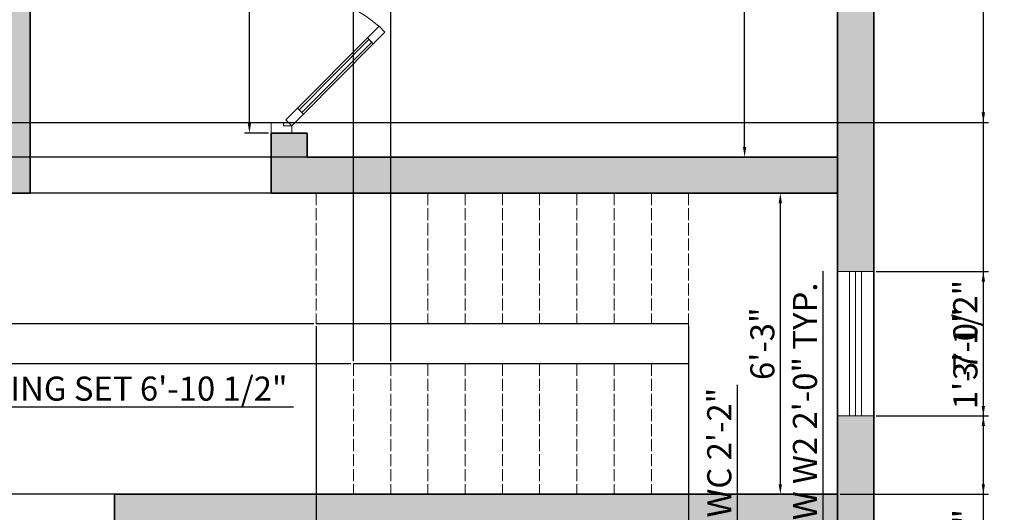
# Model space of a CAD drawing. Units: inches. Extents: x -40 to 424, y -33 to 568.
# Tile 7 of 8: x 171 to 417, y 275 to 397. Entities that reach past the tile are written whole.
import ezdxf

# ---------------------------------------------------------------- set-up
doc = ezdxf.new("R2010")
doc.units = ezdxf.units.IN
doc.linetypes.add('ACAD_ISO02W100', pattern=[15, 12, -3])
for name, color, linetype, lineweight in [('A-ANNO-DIMS', 7, 'Continuous', 18), ('A-DOOR', 7, 'Continuous', 18), ('A-FLOR-STRS', 7, 'Continuous', 25), ('A-FLOR-STRS-OVHD', 7, 'ACAD_ISO02W100', 18), ('A-GLAZ', 7, 'Continuous', 18), ('A-WALL-OVHD', 7, 'ACAD_ISO02W100', 18), ('A-WALL-PATT', 30, 'Continuous', 13), ('wall', 7, 'Continuous', 35)]:
    doc.layers.add(name, color=color, linetype=linetype, lineweight=lineweight)
doc.styles.get("Standard").update_dxf_attribs({"font": 'arial.ttf'})
doc.dimstyles.new('ISO-25', dxfattribs={"dimtxt": 6, "dimasz": 2.5, "dimexe": 1.25, "dimexo": 0.625, "dimtad": 1, "dimdec": 1, "dimlunit": 3, "dimtxsty": 'Standard', "dimcen": 2.5, "dimadec": 0, "dimazin": 0, "dimtfac": 1, "dimtdec": 1, "dimtmove": 0, "dimatfit": 3, "dimfxl": 1, "dimarcsym": 0})

# ---------------------------------------------------------------- blocks, each defined once
blk = doc.blocks.new('A$C3C032968')
for p, q in [((0, 0), (0, 100)), ((0, 100), (0, 0)), ((700, 0), (700, 100)), ((700, 0), (700, 100))]:
    blk.add_line(p, q)
for points in [[(517.5, 522.4), (460.7, 466.1), (432.5, 494.5), (489.3, 550.8)], [(120, 128), (460.7, 466.1), (432.5, 494.5), (91.8, 156.4)], [(112.9, 135.1), (453.6, 473.2), (439.5, 487.4), (98.8, 149.3)], [(63.2, 71.6), (120, 128), (91.8, 156.4), (35, 100)], [(35, 100), (0, 100), (0, 0), (50, 0), (50, 50), (50, 60), (35, 60)], [(665, 100), (665, 60), (650, 60), (650, 50), (650, 0), (700, 0), (700, 100)]]:
    blk.add_lwpolyline(points, close=True)
blk.add_arc((72.4, 128.7), 593.3, 357.2313, 41.4937)
blk = doc.blocks.new('*D34')
at = {"layer": 'A-ANNO-DIMS', "color": 0, "lineweight": -2, "transparency": 16777216}
for p, q in [((353.15, 519), (350.62, 519)), ((351.87, 365.5), (351.87, 516.5)), ((353.15, 363), (350.62, 363))]:
    blk.add_line(p, q, dxfattribs=at)
at = {"layer": 'A-ANNO-DIMS', "color": 0, "transparency": 16777216}
for points in [[(351.46, 516.5), (352.29, 516.5), (351.87, 519)], [(351.46, 365.5), (352.29, 365.5), (351.87, 363)]]:
    blk.add_solid(points, dxfattribs=at)
at = {"layer": 'Defpoints', "color": 0, "transparency": 16777216}
for p in [(351.87, 519), (353.78, 519), (353.78, 363)]:
    blk.add_point(p, dxfattribs=at)
at = {"layer": 'A-ANNO-DIMS', "color": 0, "transparency": 16777216, "insert": (348.18, 441), "char_height": 6, "attachment_point": 5, "rotation": 90}
blk.add_mtext("13'", dxfattribs=at)
blk = doc.blocks.new('*D35')
at = {"layer": 'A-ANNO-DIMS', "color": 0, "lineweight": -2, "transparency": 16777216}
for p, q in [((352.5, 354), (362.01, 354)), ((360.76, 351.5), (360.76, 281.5)), ((352.5, 279), (362.01, 279))]:
    blk.add_line(p, q, dxfattribs=at)
at = {"layer": 'A-ANNO-DIMS', "color": 0, "transparency": 16777216}
for points in [[(360.34, 351.5), (361.17, 351.5), (360.76, 354)], [(360.34, 281.5), (361.17, 281.5), (360.76, 279)]]:
    blk.add_solid(points, dxfattribs=at)
at = {"layer": 'Defpoints', "color": 0, "transparency": 16777216}
for p in [(351.87, 354), (351.87, 279), (360.76, 279)]:
    blk.add_point(p, dxfattribs=at)
at = {"layer": 'A-ANNO-DIMS', "color": 0, "transparency": 16777216, "insert": (357.07, 316.5), "char_height": 6, "attachment_point": 5, "rotation": 90}
blk.add_mtext('6\'-3"', dxfattribs=at)
blk = doc.blocks.new('*D45')
at = {"layer": 'A-ANNO-DIMS', "color": 0, "lineweight": -2, "transparency": 16777216}
for p, q in [((371.4, 240), (371.4, 334.58)), ((374.38, 240), (370.15, 240)), ((371.4, 218.5), (371.4, 237.5)), ((374.38, 216), (370.15, 216))]:
    blk.add_line(p, q, dxfattribs=at)
at = {"layer": 'A-ANNO-DIMS', "color": 0, "transparency": 16777216}
for points in [[(370.98, 237.5), (371.82, 237.5), (371.4, 240)], [(370.98, 218.5), (371.82, 218.5), (371.4, 216)]]:
    blk.add_solid(points, dxfattribs=at)
at = {"layer": 'Defpoints', "color": 0, "transparency": 16777216}
for p in [(371.4, 240), (375, 240), (375, 216)]:
    blk.add_point(p, dxfattribs=at)
at = {"layer": 'A-ANNO-DIMS', "color": 0, "transparency": 16777216, "insert": (367.67, 288.54), "char_height": 6, "attachment_point": 5, "rotation": 90}
blk.add_mtext('WINDOW W2 2\'-0" TYP.', dxfattribs=at)
blk = doc.blocks.new('*D47')
at = {"layer": 'A-ANNO-DIMS', "color": 0, "lineweight": -2, "transparency": 16777216}
for p, q in [((228.6, 405), (228.6, 472.5)), ((233.37, 405), (227.35, 405)), ((228.6, 371.5), (228.6, 402.5)), ((233.37, 369), (227.35, 369))]:
    blk.add_line(p, q, dxfattribs=at)
at = {"layer": 'A-ANNO-DIMS', "color": 0, "transparency": 16777216}
for points in [[(228.18, 402.5), (229.02, 402.5), (228.6, 405)], [(228.18, 371.5), (229.02, 371.5), (228.6, 369)]]:
    blk.add_solid(points, dxfattribs=at)
at = {"layer": 'Defpoints', "color": 0, "transparency": 16777216}
for p in [(228.6, 405), (234, 405), (234, 369)]:
    blk.add_point(p, dxfattribs=at)
at = {"layer": 'A-ANNO-DIMS', "color": 0, "transparency": 16777216, "insert": (224.87, 440), "char_height": 6, "attachment_point": 5, "rotation": 90}
blk.add_mtext('DOOR 3\'-0" TYP.', dxfattribs=at)
blk = doc.blocks.new('*D61')
at = {"layer": 'A-ANNO-DIMS', "color": 0, "lineweight": -2, "transparency": 16777216}
for p, q in [((68.52, 312.6), (68.52, 299.57)), ((151.21, 312.6), (151.21, 299.57)), ((71.02, 300.82), (148.71, 300.82)), ((151.21, 300.82), (239.55, 300.82))]:
    blk.add_line(p, q, dxfattribs=at)
at = {"layer": 'A-ANNO-DIMS', "color": 0, "transparency": 16777216}
for points in [[(71.02, 301.23), (71.02, 300.4), (68.52, 300.82)], [(148.71, 301.23), (148.71, 300.4), (151.21, 300.82)]]:
    blk.add_solid(points, dxfattribs=at)
at = {"layer": 'Defpoints', "color": 0, "transparency": 16777216}
for p in [(68.52, 313.22), (151.21, 313.22), (151.21, 300.82)]:
    blk.add_point(p, dxfattribs=at)
at = {"layer": 'A-ANNO-DIMS', "color": 0, "transparency": 16777216, "insert": (196.63, 304.54), "char_height": 6, "attachment_point": 5}
blk.add_mtext('DINING SET 6\'-10 1/2"', dxfattribs=at)
blk = doc.blocks.new('*D69')
at = {"layer": 'A-ANNO-DIMS', "color": 0, "lineweight": -2, "transparency": 16777216}
for p, q in [((350.07, 270), (350.07, 306.24)), ((346.8, 270), (351.32, 270)), ((350.07, 246.57), (350.07, 267.5)), ((346.8, 244.07), (351.32, 244.07))]:
    blk.add_line(p, q, dxfattribs=at)
at = {"layer": 'A-ANNO-DIMS', "color": 0, "transparency": 16777216}
for points in [[(349.65, 267.5), (350.48, 267.5), (350.07, 270)], [(349.65, 246.57), (350.48, 246.57), (350.07, 244.07)]]:
    blk.add_solid(points, dxfattribs=at)
at = {"layer": 'Defpoints', "color": 0, "transparency": 16777216}
for p in [(346.18, 270), (350.07, 270), (346.18, 244.07)]:
    blk.add_point(p, dxfattribs=at)
at = {"layer": 'A-ANNO-DIMS', "color": 0, "transparency": 16777216, "insert": (346.34, 289.37), "char_height": 6, "attachment_point": 5, "rotation": 90}
blk.add_mtext('WC 2\'-2"', dxfattribs=at)
blk = doc.blocks.new('*D80')
at = {"layer": 'A-ANNO-DIMS', "color": 0, "lineweight": -2, "transparency": 16777216}
for p, q in [((384.63, 528), (412.55, 528)), ((411.3, 2.5), (411.3, 525.5)), ((384.63, 0), (412.55, 0))]:
    blk.add_line(p, q, dxfattribs=at)
at = {"layer": 'A-ANNO-DIMS', "color": 0, "transparency": 16777216}
for points in [[(410.88, 525.5), (411.72, 525.5), (411.3, 528)], [(410.88, 2.5), (411.72, 2.5), (411.3, 0)]]:
    blk.add_solid(points, dxfattribs=at)
at = {"layer": 'Defpoints', "color": 0, "transparency": 16777216}
for p in [(384, 528), (411.3, 528), (384, 0)]:
    blk.add_point(p, dxfattribs=at)
at = {"layer": 'A-ANNO-DIMS', "color": 0, "transparency": 16777216, "insert": (407.61, 264), "char_height": 6, "attachment_point": 5, "rotation": 90}
blk.add_mtext('44\'-0"', dxfattribs=at)
blk = doc.blocks.new('*D89')
at = {"layer": 'A-ANNO-DIMS', "color": 0, "lineweight": -2, "transparency": 16777216}
for p, q in [((374.38, 417), (-28.55, 417)), ((-27.3, 365.5), (-27.3, 414.5)), ((374.38, 363), (-28.55, 363))]:
    blk.add_line(p, q, dxfattribs=at)
at = {"layer": 'A-ANNO-DIMS', "color": 0, "transparency": 16777216}
for points in [[(-27.72, 414.5), (-26.88, 414.5), (-27.3, 417)], [(-27.72, 365.5), (-26.88, 365.5), (-27.3, 363)]]:
    blk.add_solid(points, dxfattribs=at)
at = {"layer": 'Defpoints', "color": 0, "transparency": 16777216}
for p in [(-27.3, 417), (375, 417), (375, 363)]:
    blk.add_point(p, dxfattribs=at)
at = {"layer": 'A-ANNO-DIMS', "color": 0, "transparency": 16777216, "insert": (-30.99, 390), "char_height": 6, "attachment_point": 5, "rotation": 90}
blk.add_mtext('4\'-6"', dxfattribs=at)
blk = doc.blocks.new('*D93')
at = {"layer": 'A-ANNO-DIMS', "color": 0, "lineweight": -2, "transparency": 16777216}
for p, q in [((411.3, 298.5), (411.3, 331.62)), ((384.63, 298.5), (412.55, 298.5)), ((411.3, 281.5), (411.3, 296)), ((375.63, 279), (412.55, 279))]:
    blk.add_line(p, q, dxfattribs=at)
at = {"layer": 'A-ANNO-DIMS', "color": 0, "transparency": 16777216}
for points in [[(410.88, 296), (411.72, 296), (411.3, 298.5)], [(410.88, 281.5), (411.72, 281.5), (411.3, 279)]]:
    blk.add_solid(points, dxfattribs=at)
at = {"layer": 'Defpoints', "color": 0, "transparency": 16777216}
for p in [(384, 298.5), (411.3, 298.5), (375, 279)]:
    blk.add_point(p, dxfattribs=at)
at = {"layer": 'A-ANNO-DIMS', "color": 0, "transparency": 16777216, "insert": (407.57, 316.31), "char_height": 6, "attachment_point": 5, "rotation": 90}
blk.add_mtext('1\'-7 1/2"', dxfattribs=at)
blk = doc.blocks.new('*D94')
at = {"layer": 'A-ANNO-DIMS', "color": 0, "lineweight": -2, "transparency": 16777216}
for p, q in [((384.63, 334.5), (412.55, 334.5)), ((411.3, 301), (411.3, 332)), ((384.63, 298.5), (412.55, 298.5))]:
    blk.add_line(p, q, dxfattribs=at)
at = {"layer": 'A-ANNO-DIMS', "color": 0, "transparency": 16777216}
for points in [[(410.88, 332), (411.72, 332), (411.3, 334.5)], [(410.88, 301), (411.72, 301), (411.3, 298.5)]]:
    blk.add_solid(points, dxfattribs=at)
at = {"layer": 'Defpoints', "color": 0, "transparency": 16777216}
for p in [(384, 334.5), (411.3, 334.5), (384, 298.5)]:
    blk.add_point(p, dxfattribs=at)
at = {"layer": 'A-ANNO-DIMS', "color": 0, "transparency": 16777216, "insert": (407.61, 316.5), "char_height": 6, "attachment_point": 5, "rotation": 90}
blk.add_mtext('3\'-0"', dxfattribs=at)
blk = doc.blocks.new('*D95')
at = {"layer": 'A-ANNO-DIMS', "color": 0, "lineweight": -2, "transparency": 16777216}
for p, q in [((375, 333.88), (375, -28.55)), ((337.92, 320.88), (337.92, -28.55)), ((340.42, -27.3), (372.5, -27.3))]:
    blk.add_line(p, q, dxfattribs=at)
at = {"layer": 'A-ANNO-DIMS', "color": 0, "transparency": 16777216}
for points in [[(340.42, -26.88), (340.42, -27.72), (337.92, -27.3)], [(372.5, -26.88), (372.5, -27.72), (375, -27.3)]]:
    blk.add_solid(points, dxfattribs=at)
at = {"layer": 'Defpoints', "color": 0, "transparency": 16777216}
for p in [(375, 334.5), (337.92, 321.5), (375, -27.3)]:
    blk.add_point(p, dxfattribs=at)
at = {"layer": 'A-ANNO-DIMS', "color": 0, "transparency": 16777216, "insert": (356.46, -23.61), "char_height": 6, "attachment_point": 5}
blk.add_mtext('3\'-1"', dxfattribs=at)
blk = doc.blocks.new('*D96')
at = {"layer": 'A-ANNO-DIMS', "color": 0, "lineweight": -2, "transparency": 16777216}
for p, q in [((245.23, 320.88), (245.23, -28.55)), ((337.92, 320.88), (337.92, -28.55)), ((247.73, -27.3), (335.42, -27.3))]:
    blk.add_line(p, q, dxfattribs=at)
at = {"layer": 'A-ANNO-DIMS', "color": 0, "transparency": 16777216}
for points in [[(247.73, -26.88), (247.73, -27.72), (245.23, -27.3)], [(335.42, -26.88), (335.42, -27.72), (337.92, -27.3)]]:
    blk.add_solid(points, dxfattribs=at)
at = {"layer": 'Defpoints', "color": 0, "transparency": 16777216}
for p in [(245.23, 321.5), (337.92, 321.5), (337.92, -27.3)]:
    blk.add_point(p, dxfattribs=at)
at = {"layer": 'A-ANNO-DIMS', "color": 0, "transparency": 16777216, "insert": (291.58, -23.57), "char_height": 6, "attachment_point": 5}
blk.add_mtext('7\'-8 1/2"', dxfattribs=at)
blk = doc.blocks.new('*D97')
at = {"layer": 'A-ANNO-DIMS', "color": 0, "lineweight": -2, "transparency": 16777216}
for p, q in [((253.88, 311.5), (-28.55, 311.5)), ((-27.3, 281.5), (-27.3, 309)), ((253.88, 279), (-28.55, 279))]:
    blk.add_line(p, q, dxfattribs=at)
at = {"layer": 'A-ANNO-DIMS', "color": 0, "transparency": 16777216}
for points in [[(-27.72, 309), (-26.88, 309), (-27.3, 311.5)], [(-27.72, 281.5), (-26.88, 281.5), (-27.3, 279)]]:
    blk.add_solid(points, dxfattribs=at)
at = {"layer": 'Defpoints', "color": 0, "transparency": 16777216}
for p in [(-27.3, 311.5), (254.5, 311.5), (254.5, 279)]:
    blk.add_point(p, dxfattribs=at)
at = {"layer": 'A-ANNO-DIMS', "color": 0, "transparency": 16777216, "insert": (-31.03, 295.25), "char_height": 6, "attachment_point": 5, "rotation": 90}
blk.add_mtext('2\'-8 1/2"', dxfattribs=at)
blk = doc.blocks.new('*D98')
at = {"layer": 'A-ANNO-DIMS', "color": 0, "lineweight": -2, "transparency": 16777216}
for p, q in [((254.5, 312.12), (254.5, 556.55)), ((263.77, 312.12), (263.77, 556.55)), ((257, 555.3), (261.27, 555.3)), ((263.77, 555.3), (297.45, 555.3))]:
    blk.add_line(p, q, dxfattribs=at)
at = {"layer": 'A-ANNO-DIMS', "color": 0, "transparency": 16777216}
for points in [[(257, 555.72), (257, 554.88), (254.5, 555.3)], [(261.27, 555.72), (261.27, 554.88), (263.77, 555.3)]]:
    blk.add_solid(points, dxfattribs=at)
at = {"layer": 'Defpoints', "color": 0, "transparency": 16777216}
for p in [(263.77, 555.3), (254.5, 311.5), (263.77, 311.5)]:
    blk.add_point(p, dxfattribs=at)
at = {"layer": 'A-ANNO-DIMS', "color": 0, "transparency": 16777216, "insert": (281.86, 559.03), "char_height": 6, "attachment_point": 5}
blk.add_mtext('0\'-9 1/2"', dxfattribs=at)
blk = doc.blocks.new('*D99')
at = {"layer": 'A-ANNO-DIMS', "color": 0, "lineweight": -2, "transparency": 16777216}
for p, q in [((244.61, 354), (-28.55, 354)), ((-27.3, 324), (-27.3, 351.5)), ((244.61, 321.5), (-28.55, 321.5))]:
    blk.add_line(p, q, dxfattribs=at)
at = {"layer": 'A-ANNO-DIMS', "color": 0, "transparency": 16777216}
for points in [[(-27.72, 351.5), (-26.88, 351.5), (-27.3, 354)], [(-27.72, 324), (-26.88, 324), (-27.3, 321.5)]]:
    blk.add_solid(points, dxfattribs=at)
at = {"layer": 'Defpoints', "color": 0, "transparency": 16777216}
for p in [(-27.3, 354), (245.23, 354), (245.23, 321.5)]:
    blk.add_point(p, dxfattribs=at)
at = {"layer": 'A-ANNO-DIMS', "color": 0, "transparency": 16777216, "insert": (-31.03, 337.75), "char_height": 6, "attachment_point": 5, "rotation": 90}
blk.add_mtext('2\'-8 1/2"', dxfattribs=at)
blk = doc.blocks.new('*D103')
at = {"layer": 'A-ANNO-DIMS', "color": 0, "lineweight": -2, "transparency": 16777216}
for p, q in [((411.3, 402.13), (411.3, 435.91)), ((34.13, 402.13), (412.55, 402.13)), ((411.3, 374.13), (411.3, 399.63)), ((34.13, 371.63), (412.55, 371.63))]:
    blk.add_line(p, q, dxfattribs=at)
at = {"layer": 'A-ANNO-DIMS', "color": 0, "transparency": 16777216}
for points in [[(410.88, 399.63), (411.72, 399.63), (411.3, 402.13)], [(410.88, 374.13), (411.72, 374.13), (411.3, 371.63)]]:
    blk.add_solid(points, dxfattribs=at)
at = {"layer": 'Defpoints', "color": 0, "transparency": 16777216}
for p in [(33.5, 402.13), (411.3, 402.13), (33.5, 371.63)]:
    blk.add_point(p, dxfattribs=at)
at = {"layer": 'A-ANNO-DIMS', "color": 0, "transparency": 16777216, "insert": (407.57, 420.27), "char_height": 6, "attachment_point": 5, "rotation": 90}
blk.add_mtext('2\'-6 1/2"', dxfattribs=at)

msp = doc.modelspace()

# ---------------------------------------------------------------- hatches: boundary and pattern name
at = {"layer": 'A-WALL-PATT'}
h = msp.add_hatch(color=256, dxfattribs=at)
h.dxf.hatch_style = 1
h.paths.add_polyline_path([(9, 399), (0, 399), (0, 351), (9, 351)])
h.paths.add_polyline_path([(9, 303), (0, 303), (0, 210), (9, 210)])
h.paths.add_polyline_path([(9, 150), (0, 150), (0, 0), (384, 0), (384, 69), (375, 69), (375, 62.24), (375, 9), (9, 9)])
h.paths.add_polyline_path([(210, 177), (216, 177), (216, 186), (210, 186), (210, 216), (201, 216), (201, 90), (195, 90), (195, 81), (201, 81), (201, 9), (210, 9)])
h.paths.add_polyline_path([(384, 216), (375, 216), (375, 117), (384, 117)])
h.paths.add_polyline_path([(384, 298.5), (375, 298.5), (375, 279), (375, 240), (384, 240)])
h.paths.add_polyline_path([(384, 417), (375, 417), (375, 334.5), (384, 334.5)])
h.paths.add_polyline_path([(384, 528), (216, 528), (216, 519), (375, 519), (375, 465), (384, 465)])
h.paths.add_polyline_path([(192, 528), (0, 528), (0, 511.5), (9, 511.5), (9, 519), (192, 519)])
h.paths.add_polyline_path([(9, 487.5), (0, 487.5), (0, 447), (9, 447)])
h.paths.add_polyline_path([(111, 480), (9, 480), (9, 471), (111, 471)])
h.paths.add_polyline_path([(174, 519), (165, 519), (165, 354), (174, 354)])
h.paths.add_polyline_path([(243, 426), (237.86, 426), (234, 426), (234, 420), (174, 420), (174, 411), (234, 411), (234, 405), (239.14, 405), (243, 405)])
h.paths.add_polyline_path([(243, 519), (234, 519), (234, 460.14, -0.031638), (237.86, 460.2), (237.86, 462), (243, 462)])
h.paths.add_polyline_path([(243, 369), (234, 369), (234, 354), (375, 354), (375, 363), (243, 363)])
h.paths.add_polyline_path([(375, 279), (195, 279), (195, 270), (201, 270), (201, 264), (210, 264), (210, 270), (375, 270)])
h.paths.add_polyline_path([(291, 270), (282, 270), (282, 222), (286.29, 222), (291, 222)])
h.paths.add_polyline_path([(375, 186), (291, 186), (291, 192), (282, 192), (282, 186), (252, 186), (252, 180.86), (252, 177), (375, 177)])
h.paths.add_polyline_path([(147, 279), (9, 279), (9, 270), (147, 270)])

# ---------------------------------------------------------------- linework, layer by layer
at = {"layer": 'A-FLOR-STRS'}
for p, q in [((375, 354), (375, 279)), ((337.92, 321.5), (245.23, 321.5)), ((337.92, 311.5), (254.5, 311.5))]:
    msp.add_line(p, q, dxfattribs=at)
at = {"layer": 'A-FLOR-STRS-OVHD', "ltscale": 0.25}
for p, q in [((245.23, 354), (245.23, 321.5)), ((254.5, 354), (254.5, 321.5)), ((263.77, 354), (263.77, 321.5)), ((273.04, 354), (273.04, 321.5)), ((282.31, 354), (282.31, 321.5)), ((291.58, 354), (291.58, 321.5)), ((300.85, 354), (300.85, 321.5)), ((310.12, 354), (310.12, 321.5)), ((319.39, 354), (319.39, 321.5)), ((328.66, 354), (328.66, 321.5)), ((337.92, 354), (337.92, 321.5)), ((337.92, 321.5), (337.92, 279)), ((254.5, 311.5), (254.5, 279)), ((263.77, 311.5), (263.77, 279)), ((273.04, 311.5), (273.04, 279)), ((282.31, 311.5), (282.31, 279)), ((291.58, 311.5), (291.58, 279)), ((300.85, 311.5), (300.85, 279)), ((310.12, 311.5), (310.12, 279)), ((319.39, 311.5), (319.39, 279)), ((328.66, 311.5), (328.66, 279))]:
    msp.add_line(p, q, dxfattribs=at)
at = {"layer": 'A-GLAZ'}
for p, q in [((375, 334.5), (384, 334.5)), ((378, 334.5), (378, 298.5)), ((379.5, 334.5), (379.5, 298.5)), ((381, 334.5), (381, 298.5)), ((375, 298.5), (384, 298.5))]:
    msp.add_line(p, q, dxfattribs=at)
at = {"layer": 'A-WALL-OVHD'}
msp.add_line((195, 279), (147, 279), dxfattribs=at)
at = {"layer": 'wall'}
for p, q in [((174, 519), (174, 354)), ((375, 9), (375, 519)), ((243, 369), (234, 369)), ((234, 369), (234, 354)), ((243, 369), (243, 363)), ((375, 363), (243, 363)), ((174, 354), (165, 354)), ((375, 354), (234, 354)), ((195, 279), (195, 270)), ((195, 279), (375, 279))]:
    msp.add_line(p, q, dxfattribs=at)
msp.add_lwpolyline([(0, 0), (384, 0), (384, 528), (0, 528)], close=True, dxfattribs=at)

# ---------------------------------------------------------------- block references
at = {"layer": 'A-DOOR', "xscale": -0.0514285714285714, "yscale": 0.0514285714285714, "zscale": 0.0514285714285714, "rotation": 269.9999999999998}
msp.add_blockref('A$C3C032968', (234, 369), dxfattribs=at)

# ---------------------------------------------------------------- dimensions: what is measured, and where the dimension line sits
at = {"layer": 'A-ANNO-DIMS'}
for base, p1, p2, picture, middle in [((263.77, 555.3), (254.5, 311.5), (263.77, 311.5), '*D98', (281.86, 559.03)), ((375, -27.3), (337.92, 321.5), (375, 334.5), '*D95', (356.46, -23.61)), ((337.92, -27.3), (245.23, 321.5), (337.92, 321.5), '*D96', (291.58, -23.57))]:
    dim = msp.add_linear_dim(base=base, p1=p1, p2=p2, dimstyle='ISO-25', override={"dimdec": 1, "dimlfac": 1, "dimrnd": 0, "dimzin": 1, "dimdsep": 46, "dimlunit": 4, "dimfrac": 2}, dxfattribs=at)
    dim.commit()
    dim.dimension.update_dxf_attribs({"geometry": picture, "text_midpoint": middle})
for base, p1, p2, override, picture, middle in [((411.3, 528), (384, 0), (384, 528), {"dimdec": 1, "dimlfac": 1, "dimrnd": 0, "dimzin": 1, "dimdsep": 46, "dimlunit": 4, "dimfrac": 2}, '*D80', (407.61, 264)), ((351.87, 519), (353.78, 363), (353.78, 519), {"dimclrd": 0, "dimclre": 0, "dimclrt": 0}, '*D34', (348.18, 441)), ((411.3, 402.13), (33.5, 371.63), (33.5, 402.13), {"dimdec": 1, "dimlfac": 1, "dimrnd": 0, "dimzin": 1, "dimdsep": 46, "dimlunit": 4, "dimfrac": 2}, '*D103', (407.57, 420.27)), ((-27.3, 417), (375, 363), (375, 417), {"dimdec": 1, "dimlfac": 1, "dimrnd": 0, "dimzin": 1, "dimdsep": 46, "dimlunit": 4, "dimfrac": 2}, '*D89', (-30.99, 390)), ((-27.3, 354), (245.23, 321.5), (245.23, 354), {"dimdec": 1, "dimlfac": 1, "dimrnd": 0, "dimzin": 1, "dimdsep": 46, "dimlunit": 4, "dimfrac": 2}, '*D99', (-31.03, 337.75)), ((360.76, 279), (351.87, 354), (351.87, 279), {"dimclrd": 0, "dimclre": 0, "dimclrt": 0}, '*D35', (357.07, 316.5)), ((411.3, 334.5), (384, 298.5), (384, 334.5), {"dimdec": 1, "dimlfac": 1, "dimrnd": 0, "dimzin": 1, "dimdsep": 46, "dimlunit": 4, "dimfrac": 2}, '*D94', (407.61, 316.5)), ((411.3, 298.5), (375, 279), (384, 298.5), {"dimdec": 1, "dimlfac": 1, "dimrnd": 0, "dimzin": 1, "dimdsep": 46, "dimlunit": 4, "dimfrac": 2}, '*D93', (407.57, 316.31)), ((-27.3, 311.5), (254.5, 279), (254.5, 311.5), {"dimdec": 1, "dimlfac": 1, "dimrnd": 0, "dimzin": 1, "dimdsep": 46, "dimlunit": 4, "dimfrac": 2}, '*D97', (-31.03, 295.25))]:
    dim = msp.add_linear_dim(base=base, p1=p1, p2=p2, angle=90, dimstyle='ISO-25', override=override, dxfattribs=at)
    dim.commit()
    dim.dimension.update_dxf_attribs({"geometry": picture, "text_midpoint": middle})
for base, p1, p2, text, picture, middle in [((228.6, 405), (234, 369), (234, 405), 'DOOR <> TYP.', '*D47', (224.87, 440)), ((371.4, 240), (375, 216), (375, 240), 'WINDOW W2 <> TYP.', '*D45', (367.67, 288.54)), ((350.07, 270), (346.18, 244.07), (346.18, 270), 'WC <>', '*D69', (346.34, 289.37))]:
    dim = msp.add_linear_dim(base=base, p1=p1, p2=p2, angle=90, text=text, dimstyle='ISO-25', override={"dimdec": 1, "dimlfac": 1, "dimrnd": 0, "dimzin": 1, "dimdsep": 46, "dimlunit": 4, "dimfrac": 2}, dxfattribs=at)
    dim.commit()
    dim.dimension.update_dxf_attribs({"geometry": picture, "text_midpoint": middle})
dim = msp.add_linear_dim(base=(151.21, 300.82), p1=(68.52, 313.22), p2=(151.21, 313.22), text='DINING SET <>', dimstyle='ISO-25', override={"dimdec": 1, "dimlfac": 1, "dimrnd": 0, "dimzin": 1, "dimdsep": 46, "dimlunit": 4, "dimfrac": 2}, dxfattribs=at)
dim.commit()
dim.dimension.update_dxf_attribs({"geometry": '*D61', "text_midpoint": (196.63, 304.54)})

doc.saveas('drawing.dxf')
